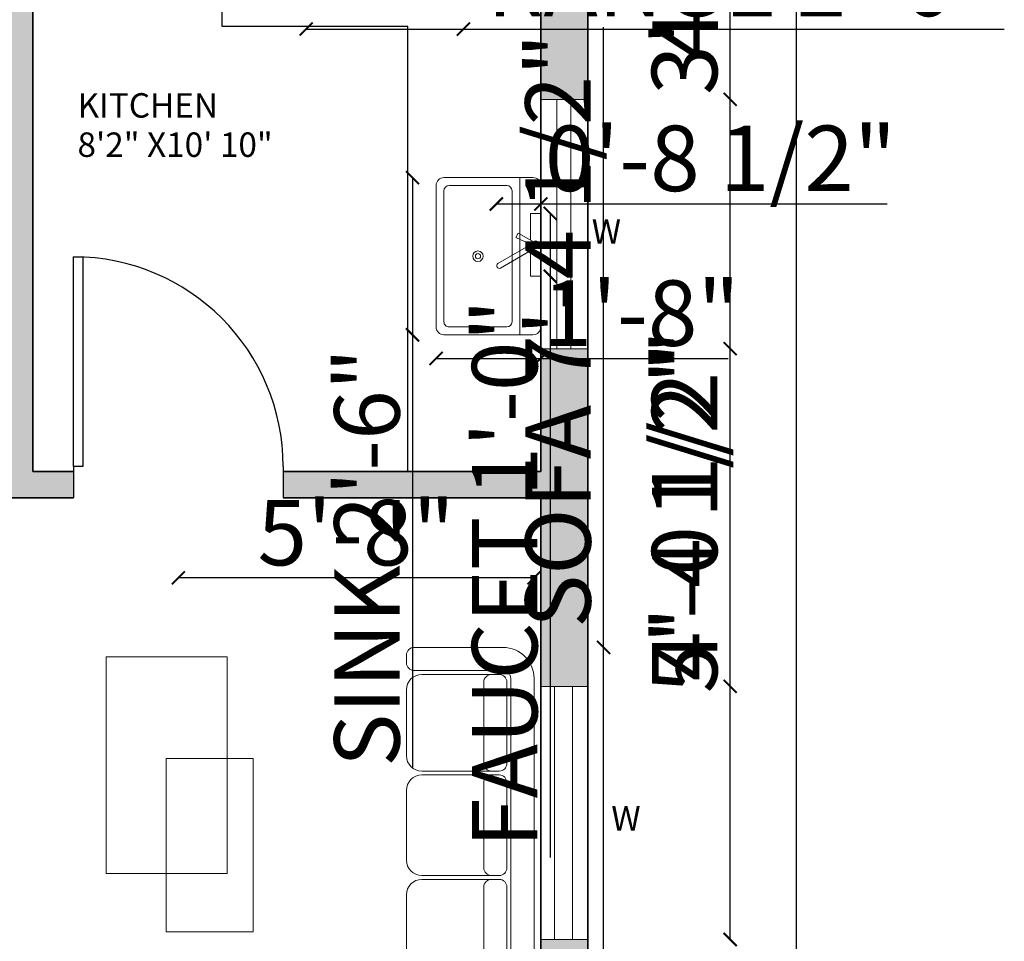
# Model space of a CAD drawing. Units: inches. Extents: x 1750 to 7466, y 1409 to 2004.
# Tile 4 of 5: x 1986 to 2174, y 1715 to 1890. Entities that reach past the tile are written whole.
import ezdxf

# ---------------------------------------------------------------- set-up
doc = ezdxf.new("R2010")
doc.units = ezdxf.units.IN
for name, color, linetype, lineweight in [('A-ANNO-DIMS', 2, 'Continuous', 18), ('A-ANNO-TEXT', 7, 'Continuous', 18), ('A-AREA-IDEN', 7, 'Continuous', 18), ('A-DOOR', 3, 'Continuous', 25), ('A-FLOR-CASE', 8, 'Continuous', 25), ('A-FLOR-FIXT', 9, 'Continuous', 18), ('A-FURN', 8, 'Continuous', 18), ('A-WALL', 7, 'Continuous', 35), ('WINDOW', 4, 'Continuous', 18)]:
    doc.layers.add(name, color=color, linetype=linetype, lineweight=lineweight)
doc.layers.add('A-WALL-PATT', color=18, linetype='Continuous', lineweight=13, true_color=0x000000)
doc.styles.get("Standard").update_dxf_attribs({"font": 'arial.ttf'})
doc.dimstyles.new('ISO-25', dxfattribs={"dimtxt": 12.5, "dimasz": 2.5, "dimexe": 1.25, "dimexo": 0.625, "dimtad": 1, "dimdec": 0, "dimlunit": 4, "dimtxsty": 'Standard', "dimblk": 'ARCHTICK', "dimcen": 2.5, "dimse1": 1, "dimse2": 1, "dimclrd": 2, "dimadec": 0, "dimazin": 0, "dimtfac": 1, "dimtdec": 0, "dimtmove": 0, "dimatfit": 3, "dimfxl": 1, "dimarcsym": 0})

# ---------------------------------------------------------------- blocks, each defined once
blk = doc.blocks.new('A$C2AFA021D')
for p, q in [((0.8, 2.3), (0.2, 2.3)), ((0.85, 2.2), (0.85, 2.25)), ((0.2, 2.15), (0.8, 2.15)), ((0.225, 2.125), (0.275, 2.125)), ((0.75, 2.125), (0.275, 2.125)), ((0, 2.1), (0, 0.2)), ((0.15, 0.2), (0.15, 2.1)), ((0.175, 1.55), (0.175, 2.075)), ((0.325, 2.075), (0.325, 1.55)), ((0.85, 1.6), (0.85, 2.025)), ((0.275, 1.5), (0.225, 1.5)), ((0.225, 1.475), (0.275, 1.475)), ((0.275, 1.5), (0.75, 1.5)), ((0.75, 1.475), (0.275, 1.475)), ((0.175, 0.875), (0.175, 1.425)), ((0.325, 1.425), (0.325, 0.875)), ((0.85, 0.925), (0.85, 1.375)), ((0.275, 0.825), (0.225, 0.825)), ((0.225, 0.8), (0.275, 0.8)), ((0.275, 0.825), (0.75, 0.825)), ((0.75, 0.8), (0.275, 0.8)), ((0.975, 0.825), (1.4, 0.825)), ((1.625, 0.825), (2.075, 0.825)), ((2.3, 0.825), (2.725, 0.825)), ((2.85, 0.2), (2.85, 0.775)), ((2.9, 0.825), (2.95, 0.825)), ((3, 0.775), (3, 0.2)), ((0.175, 0.225), (0.175, 0.75)), ((0.325, 0.75), (0.325, 0.225)), ((0.875, 0.275), (0.875, 0.725)), ((1.5, 0.725), (1.5, 0.275)), ((1.525, 0.275), (1.525, 0.725)), ((2.175, 0.725), (2.175, 0.275)), ((2.2, 0.275), (2.2, 0.725)), ((2.825, 0.725), (2.825, 0.275)), ((0.85, 0.275), (0.85, 0.7)), ((1.45, 0.325), (0.925, 0.325)), ((2.125, 0.325), (1.575, 0.325)), ((2.775, 0.325), (2.25, 0.325)), ((0.875, 0.275), (0.875, 0.225)), ((1.5, 0.225), (1.5, 0.275)), ((1.525, 0.275), (1.525, 0.225)), ((2.175, 0.225), (2.175, 0.275)), ((2.2, 0.275), (2.2, 0.225)), ((2.825, 0.225), (2.825, 0.275)), ((0.8, 0.15), (0.2, 0.15)), ((0.275, 0.175), (0.225, 0.175)), ((0.275, 0.175), (0.75, 0.175)), ((0.925, 0.175), (1.45, 0.175)), ((0.925, 0.15), (2.8, 0.15)), ((1.575, 0.175), (2.125, 0.175)), ((2.25, 0.175), (2.775, 0.175)), ((0.85, 0), (0.85, 0.1)), ((0.875, 0.1), (0.875, 0)), ((0.2, 0), (0.85, 0)), ((2.8, 0), (0.875, 0))]:
    blk.add_line(p, q)
for centre, radius, start, end in [((0.2, 2.1), 0.2, 90, 180), ((0.8, 2.25), 0.05, 0, 90), ((0.8, 2.2), 0.05, 270, 0), ((0.2, 2.1), 0.05, 90, 180), ((0.225, 2.075), 0.05, 90, 180), ((0.275, 2.075), 0.05, 0, 90), ((0.75, 2.025), 0.1, 0, 90), ((0.75, 1.6), 0.1, 270, 0), ((0.225, 1.55), 0.05, 180, 270), ((0.275, 1.55), 0.05, 270, 0), ((0.225, 1.425), 0.05, 90, 180), ((0.275, 1.425), 0.05, 0, 90), ((0.75, 1.375), 0.1, 360, 90), ((0.75, 0.925), 0.1, 270, 0), ((0.225, 0.875), 0.05, 180, 270), ((0.275, 0.875), 0.05, 270, 0), ((0.225, 0.75), 0.05, 90, 180), ((0.275, 0.75), 0.05, 0, 90), ((0.75, 0.7), 0.1, 0, 90), ((0.975, 0.725), 0.1, 90, 180), ((1.4, 0.725), 0.1, 0, 90), ((1.625, 0.725), 0.1, 90, 180), ((2.075, 0.725), 0.1, 0, 90), ((2.3, 0.725), 0.1, 90, 180), ((2.725, 0.725), 0.1, 0, 90), ((2.9, 0.775), 0.05, 90, 180), ((2.95, 0.775), 0.05, 0, 90), ((0.925, 0.275), 0.05, 90, 180), ((1.45, 0.275), 0.05, 360, 90), ((1.575, 0.275), 0.05, 90, 180), ((2.125, 0.275), 0.05, 360, 90), ((2.25, 0.275), 0.05, 90, 180), ((2.775, 0.275), 0.05, 360, 90), ((0.75, 0.275), 0.1, 270, 0), ((0.2, 0.2), 0.2, 180, 270), ((0.2, 0.2), 0.05, 180, 270), ((0.225, 0.225), 0.05, 180, 270), ((0.275, 0.225), 0.05, 270, 0), ((0.925, 0.225), 0.05, 180, 270), ((1.45, 0.225), 0.05, 270, 0), ((1.575, 0.225), 0.05, 180, 270), ((2.125, 0.225), 0.05, 270, 0), ((2.25, 0.225), 0.05, 180, 270), ((2.775, 0.225), 0.05, 270, 0), ((2.8, 0.2), 0.2, 270, 0), ((2.8, 0.2), 0.05, 270, 0), ((0.8, 0.1), 0.05, 0, 90), ((0.925, 0.1), 0.05, 90, 180)]:
    blk.add_arc(centre, radius, start, end)
blk = doc.blocks.new('Faucet - single handle top')
for p, q in [((0.08, -0.26), (-2.26, -4.34)), ((-1.37, -4.79), (0.55, -0.5)), ((4.43, -7.68), (0.72, -1.24)), ((-0.06, -1.9), (3.57, -8.18)), ((-2.26, -4.34), (-1.37, -4.79))]:
    blk.add_line(p, q)
for points in [[(-0.92, -2), (-6, -2), (-6, 0), (6, 0), (6, -2), (1.16, -2)], [(-0.01, -2), (-0.12, -2)]]:
    blk.add_lwpolyline(points)
for centre, radius, start, end in [((0, -1), 0.75, 269.2246, 216.2304), ((4, -7.93), 0.5, 210, 30)]:
    blk.add_arc(centre, radius, start, end)
blk = doc.blocks.new('Sink-single - 30 in top')
blk.add_line((-15, -3.999996), (15, -3.999996))
for points in [[(-13.5, 0), (13.5, 0)], [(-15, -18.499996), (-15, -1.5)], [(15, -1.5), (15, -18.499996)], [(-12.5, -5.499996), (12.5, -5.499996)], [(-13.5, -17.499996), (-13.5, -6.499996)], [(13.5, -6.499996), (13.5, -17.499996)], [(12.5, -18.499996), (-12.5, -18.499996)], [(13.5, -19.999996), (-13.5, -19.999996)]]:
    blk.add_lwpolyline(points)
for radius in [1, 0.5]:
    blk.add_circle((0, -11.999996), radius)
for centre, radius, start, end in [((-13.5, -1.5), 1.5, 90, 180), ((13.5, -1.5), 1.5, 0, 90), ((-12.5, -6.499996), 1, 90, 180), ((12.5, -6.499996), 1, 0, 90), ((-13.5, -18.499996), 1.5, 180, 270), ((-12.5, -17.499996), 1, 180, 270), ((12.5, -17.499996), 1, 270, 0), ((13.5, -18.499996), 1.5, 270, 0)]:
    blk.add_arc(centre, radius, start, end)
blk = doc.blocks.new('*U11')
for p, q in [((0, 0), (0, -6)), ((40, 0), (40, -6))]:
    blk.add_line(p, q)
blk.add_lwpolyline([(0, 0), (0, 40), (1.75, 40), (1.75, 0)], close=True)
blk.add_arc((0, 0), 40, 0, 90)
blk = doc.blocks.new('_ArchTick')
at = {"color": 0, "linetype": 'ByBlock', "const_width": 0.15}
blk.add_lwpolyline([(-0.5, -0.5), (0.5, 0.5)], dxfattribs=at)
blk = doc.blocks.new('*D14')
at = {"layer": 'A-ANNO-DIMS', "color": 0, "lineweight": -2, "transparency": 16777216}
blk.add_line((2133.87, 1928.17), (2133.87, 1448.17), dxfattribs=at)
at = {"layer": 'Defpoints', "color": 0, "transparency": 16777216}
for p in [(2094.13, 1928.17), (2094.13, 1448.17), (2133.87, 1448.17)]:
    blk.add_point(p, dxfattribs=at)
at = {"layer": 'A-ANNO-DIMS', "color": 0, "lineweight": -2, "transparency": 16777216, "xscale": 2.5, "yscale": 2.5, "zscale": 2.5}
for p, rotation in [((2133.87, 1928.17), 90), ((2133.87, 1448.17), 270)]:
    blk.add_blockref('_ArchTick', p, dxfattribs=dict(at, rotation=rotation))
at = {"layer": 'A-ANNO-DIMS', "color": 0, "transparency": 16777216, "insert": (2126.86, 1688.17), "char_height": 12.5, "attachment_point": 5, "rotation": 90}
blk.add_mtext("40'", dxfattribs=at)
blk = doc.blocks.new('*D17')
at = {"layer": 'A-ANNO-DIMS', "color": 2, "lineweight": -2, "transparency": 16777216}
for p, q in [((2097.12, 1770.61), (2097.12, 1889.05)), ((2097.12, 1682.03), (2097.12, 1770.61))]:
    blk.add_line(p, q, dxfattribs=at)
at = {"layer": 'Defpoints', "color": 0, "transparency": 16777216}
for p in [(2083.83, 1770.61), (2097.12, 1770.61), (2083.83, 1682.03)]:
    blk.add_point(p, dxfattribs=at)
at = {"layer": 'A-ANNO-DIMS', "color": 2, "lineweight": -2, "transparency": 16777216, "xscale": 2.5, "yscale": 2.5, "zscale": 2.5}
for p, rotation in [((2097.12, 1770.61), 90), ((2097.12, 1682.03), 270)]:
    blk.add_blockref('_ArchTick', p, dxfattribs=dict(at, rotation=rotation))
at = {"layer": 'A-ANNO-DIMS', "color": 0, "transparency": 16777216, "insert": (2090.03, 1831.08), "char_height": 12.5, "attachment_point": 5, "rotation": 90}
blk.add_mtext('SOFA 7\'-4 1/2"', dxfattribs=at)
blk = doc.blocks.new('*D18')
at = {"layer": 'A-ANNO-DIMS', "color": 2, "lineweight": -2, "transparency": 16777216}
blk.add_line((2083.83, 1783.9), (2015.92, 1783.9), dxfattribs=at)
at = {"layer": 'Defpoints', "color": 0, "transparency": 16777216}
for p in [(2015.92, 1783.9), (2015.92, 1770.61), (2083.83, 1770.61)]:
    blk.add_point(p, dxfattribs=at)
at = {"layer": 'A-ANNO-DIMS', "color": 2, "lineweight": -2, "transparency": 16777216, "xscale": 2.5, "yscale": 2.5, "zscale": 2.5, "rotation": 180}
blk.add_blockref('_ArchTick', (2015.92, 1783.9), dxfattribs=at)
at = {"layer": 'A-ANNO-DIMS', "color": 2, "lineweight": -2, "transparency": 16777216, "xscale": 2.5, "yscale": 2.5, "zscale": 2.5}
blk.add_blockref('_ArchTick', (2083.83, 1783.9), dxfattribs=at)
at = {"layer": 'A-ANNO-DIMS', "color": 0, "transparency": 16777216, "insert": (2049.88, 1790.91), "char_height": 12.5, "attachment_point": 5}
blk.add_mtext('5\'-8"', dxfattribs=at)
blk = doc.blocks.new('*D19')
at = {"layer": 'A-ANNO-DIMS', "color": 2, "lineweight": -2, "transparency": 16777216}
for p, q in [((2040.34, 1888.67), (2070.34, 1888.67)), ((2070.34, 1888.67), (2173.62, 1888.67))]:
    blk.add_line(p, q, dxfattribs=at)
at = {"layer": 'Defpoints', "color": 0, "transparency": 16777216}
for p in [(2040.34, 1893.17), (2070.34, 1893.17), (2070.34, 1888.67)]:
    blk.add_point(p, dxfattribs=at)
at = {"layer": 'A-ANNO-DIMS', "color": 2, "lineweight": -2, "transparency": 16777216, "xscale": 2.5, "yscale": 2.5, "zscale": 2.5, "rotation": 180}
blk.add_blockref('_ArchTick', (2040.34, 1888.67), dxfattribs=at)
at = {"layer": 'A-ANNO-DIMS', "color": 2, "lineweight": -2, "transparency": 16777216, "xscale": 2.5, "yscale": 2.5, "zscale": 2.5}
blk.add_blockref('_ArchTick', (2070.34, 1888.67), dxfattribs=at)
at = {"layer": 'A-ANNO-DIMS', "color": 0, "transparency": 16777216, "insert": (2123.23, 1895.75), "char_height": 12.5, "attachment_point": 5}
blk.add_mtext('RANGE 2\'-6"', dxfattribs=at)
blk = doc.blocks.new('*D21')
at = {"layer": 'A-ANNO-DIMS', "color": 2, "lineweight": -2, "transparency": 16777216}
for p, q in [((2060.63, 1860.3), (2060.63, 1830.3)), ((2060.63, 1830.3), (2060.63, 1747.77))]:
    blk.add_line(p, q, dxfattribs=at)
at = {"layer": 'Defpoints', "color": 0, "transparency": 16777216}
for p in [(2065.13, 1860.3), (2060.63, 1830.3), (2065.13, 1830.3)]:
    blk.add_point(p, dxfattribs=at)
at = {"layer": 'A-ANNO-DIMS', "color": 2, "lineweight": -2, "transparency": 16777216, "xscale": 2.5, "yscale": 2.5, "zscale": 2.5}
for p, rotation in [((2060.63, 1860.3), 90), ((2060.63, 1830.3), 270)]:
    blk.add_blockref('_ArchTick', p, dxfattribs=dict(at, rotation=rotation))
at = {"layer": 'A-ANNO-DIMS', "color": 0, "transparency": 16777216, "insert": (2053.55, 1787.79), "char_height": 12.5, "attachment_point": 5, "rotation": 90}
blk.add_mtext('SINK 2\'-6"', dxfattribs=at)
blk = doc.blocks.new('*D22')
at = {"layer": 'A-ANNO-DIMS', "color": 2, "lineweight": -2, "transparency": 16777216}
for p, q in [((2065.13, 1825.8), (2085.13, 1825.8)), ((2085.13, 1825.8), (2120.93, 1825.8))]:
    blk.add_line(p, q, dxfattribs=at)
at = {"layer": 'Defpoints', "color": 0, "transparency": 16777216}
for p in [(2065.13, 1830.3), (2085.13, 1830.3), (2085.13, 1825.8)]:
    blk.add_point(p, dxfattribs=at)
at = {"layer": 'A-ANNO-DIMS', "color": 2, "lineweight": -2, "transparency": 16777216, "xscale": 2.5, "yscale": 2.5, "zscale": 2.5, "rotation": 180}
blk.add_blockref('_ArchTick', (2065.13, 1825.8), dxfattribs=at)
at = {"layer": 'A-ANNO-DIMS', "color": 2, "lineweight": -2, "transparency": 16777216, "xscale": 2.5, "yscale": 2.5, "zscale": 2.5}
blk.add_blockref('_ArchTick', (2085.13, 1825.8), dxfattribs=at)
at = {"layer": 'A-ANNO-DIMS', "color": 0, "transparency": 16777216, "insert": (2104.28, 1832.81), "char_height": 12.5, "attachment_point": 5}
blk.add_mtext('1\'-8"', dxfattribs=at)
blk = doc.blocks.new('*D23')
at = {"layer": 'A-ANNO-DIMS', "color": 2, "lineweight": -2, "transparency": 16777216}
for p, q in [((2086.93, 1853.47), (2086.93, 1841.47)), ((2086.93, 1841.47), (2086.93, 1730.5))]:
    blk.add_line(p, q, dxfattribs=at)
at = {"layer": 'Defpoints', "color": 0, "transparency": 16777216}
for p in [(2085.13, 1853.47), (2085.13, 1841.47), (2086.93, 1841.47)]:
    blk.add_point(p, dxfattribs=at)
at = {"layer": 'A-ANNO-DIMS', "color": 2, "lineweight": -2, "transparency": 16777216, "xscale": 2.5, "yscale": 2.5, "zscale": 2.5}
for p, rotation in [((2086.93, 1853.47), 90), ((2086.93, 1841.47), 270)]:
    blk.add_blockref('_ArchTick', p, dxfattribs=dict(at, rotation=rotation))
at = {"layer": 'A-ANNO-DIMS', "color": 0, "transparency": 16777216, "insert": (2079.85, 1784.74), "char_height": 12.5, "attachment_point": 5, "rotation": 90}
blk.add_mtext('FAUCET 1\'-0"', dxfattribs=at)
blk = doc.blocks.new('*D24')
at = {"layer": 'A-ANNO-DIMS', "color": 2, "lineweight": -2, "transparency": 16777216}
for p, q in [((2076.63, 1855.27), (2085.13, 1855.27)), ((2085.13, 1855.27), (2151.24, 1855.27))]:
    blk.add_line(p, q, dxfattribs=at)
at = {"layer": 'Defpoints', "color": 0, "transparency": 16777216}
for p in [(2085.13, 1855.27), (2076.63, 1853.47), (2085.13, 1853.47)]:
    blk.add_point(p, dxfattribs=at)
at = {"layer": 'A-ANNO-DIMS', "color": 2, "lineweight": -2, "transparency": 16777216, "xscale": 2.5, "yscale": 2.5, "zscale": 2.5, "rotation": 180}
blk.add_blockref('_ArchTick', (2076.63, 1855.27), dxfattribs=at)
at = {"layer": 'A-ANNO-DIMS', "color": 2, "lineweight": -2, "transparency": 16777216, "xscale": 2.5, "yscale": 2.5, "zscale": 2.5}
blk.add_blockref('_ArchTick', (2085.13, 1855.27), dxfattribs=at)
at = {"layer": 'A-ANNO-DIMS', "color": 0, "transparency": 16777216, "insert": (2119.44, 1862.36), "char_height": 12.5, "attachment_point": 5}
blk.add_mtext('0\'-8 1/2"', dxfattribs=at)
blk = doc.blocks.new('*D38')
at = {"layer": 'A-ANNO-DIMS', "color": 2, "lineweight": -2, "transparency": 16777216}
for p, q in [((2024.28, 1421.02), (2059.72, 1421.02)), ((2059.72, 1421.02), (2135.75, 1421.02))]:
    blk.add_line(p, q, dxfattribs=at)
at = {"layer": 'Defpoints', "color": 0, "transparency": 16777216}
for p in [(2024.28, 1889.13), (2059.72, 1889.13), (2059.72, 1421.02)]:
    blk.add_point(p, dxfattribs=at)
at = {"layer": 'A-ANNO-DIMS', "color": 2, "lineweight": -2, "transparency": 16777216, "xscale": 2.5, "yscale": 2.5, "zscale": 2.5, "rotation": 180}
blk.add_blockref('_ArchTick', (2024.28, 1421.02), dxfattribs=at)
at = {"layer": 'A-ANNO-DIMS', "color": 2, "lineweight": -2, "transparency": 16777216, "xscale": 2.5, "yscale": 2.5, "zscale": 2.5}
blk.add_blockref('_ArchTick', (2059.72, 1421.02), dxfattribs=at)
at = {"layer": 'A-ANNO-DIMS', "color": 0, "transparency": 16777216, "insert": (2098.98, 1428.1), "char_height": 12.5, "attachment_point": 5}
blk.add_mtext('2\'-11 1/2"', dxfattribs=at)
blk = doc.blocks.new('*D39')
at = {"layer": 'A-ANNO-DIMS', "color": 2, "lineweight": -2, "transparency": 16777216}
for p, q in [((1775.98, 1919.17), (1775.98, 1889.13)), ((1775.98, 1889.13), (1775.98, 1851.94))]:
    blk.add_line(p, q, dxfattribs=at)
at = {"layer": 'Defpoints', "color": 0, "transparency": 16777216}
for p in [(2024.28, 1919.17), (1775.98, 1889.13), (2024.28, 1889.13)]:
    blk.add_point(p, dxfattribs=at)
at = {"layer": 'A-ANNO-DIMS', "color": 2, "lineweight": -2, "transparency": 16777216, "xscale": 2.5, "yscale": 2.5, "zscale": 2.5}
for p, rotation in [((1775.98, 1919.17), 90), ((1775.98, 1889.13), 270)]:
    blk.add_blockref('_ArchTick', p, dxfattribs=dict(at, rotation=rotation))
at = {"layer": 'A-ANNO-DIMS', "color": 0, "transparency": 16777216, "insert": (1768.98, 1869.28), "char_height": 12.5, "attachment_point": 5, "rotation": 90}
blk.add_mtext('2\'-6"', dxfattribs=at)
blk = doc.blocks.new('*D40')
at = {"layer": 'A-ANNO-DIMS', "color": 2, "lineweight": -2, "transparency": 16777216}
for p, q in [((2059.72, 1421.02), (2085.13, 1421.02)), ((2085.13, 1421.02), (2151.45, 1421.02))]:
    blk.add_line(p, q, dxfattribs=at)
at = {"layer": 'Defpoints', "color": 0, "transparency": 16777216}
for p in [(2059.72, 1804.17), (2085.13, 1804.17), (2085.13, 1421.02)]:
    blk.add_point(p, dxfattribs=at)
at = {"layer": 'A-ANNO-DIMS', "color": 2, "lineweight": -2, "transparency": 16777216, "xscale": 2.5, "yscale": 2.5, "zscale": 2.5, "rotation": 180}
blk.add_blockref('_ArchTick', (2059.72, 1421.02), dxfattribs=at)
at = {"layer": 'A-ANNO-DIMS', "color": 2, "lineweight": -2, "transparency": 16777216, "xscale": 2.5, "yscale": 2.5, "zscale": 2.5}
blk.add_blockref('_ArchTick', (2085.13, 1421.02), dxfattribs=at)
at = {"layer": 'A-ANNO-DIMS', "color": 0, "transparency": 16777216, "insert": (2119.54, 1428.1), "char_height": 12.5, "attachment_point": 5}
blk.add_mtext('2\'-1 1/2"', dxfattribs=at)
blk = doc.blocks.new('*D41')
at = {"layer": 'A-ANNO-DIMS', "color": 2, "lineweight": -2, "transparency": 16777216}
blk.add_line((1995.93, 1421.02), (2035.93, 1421.02), dxfattribs=at)
at = {"layer": 'Defpoints', "color": 0, "transparency": 16777216}
for p in [(1995.93, 1804.17), (2035.93, 1804.17), (2035.93, 1421.02)]:
    blk.add_point(p, dxfattribs=at)
at = {"layer": 'A-ANNO-DIMS', "color": 2, "lineweight": -2, "transparency": 16777216, "xscale": 2.5, "yscale": 2.5, "zscale": 2.5, "rotation": 180}
blk.add_blockref('_ArchTick', (1995.93, 1421.02), dxfattribs=at)
at = {"layer": 'A-ANNO-DIMS', "color": 2, "lineweight": -2, "transparency": 16777216, "xscale": 2.5, "yscale": 2.5, "zscale": 2.5}
blk.add_blockref('_ArchTick', (2035.93, 1421.02), dxfattribs=at)
at = {"layer": 'A-ANNO-DIMS', "color": 0, "transparency": 16777216, "insert": (2015.93, 1428.03), "char_height": 12.5, "attachment_point": 5}
blk.add_mtext('3\'-4"', dxfattribs=at)
blk = doc.blocks.new('*D44')
at = {"layer": 'A-ANNO-DIMS', "color": 2, "lineweight": -2, "transparency": 16777216}
for p, q in [((2121.28, 1875.24), (2121.28, 1951.04)), ((2121.28, 1827.64), (2121.28, 1875.24))]:
    blk.add_line(p, q, dxfattribs=at)
at = {"layer": 'Defpoints', "color": 0, "transparency": 16777216}
for p in [(2094.13, 1875.24), (2121.28, 1875.24), (2094.13, 1827.64)]:
    blk.add_point(p, dxfattribs=at)
at = {"layer": 'A-ANNO-DIMS', "color": 2, "lineweight": -2, "transparency": 16777216, "xscale": 2.5, "yscale": 2.5, "zscale": 2.5}
for p, rotation in [((2121.28, 1875.24), 90), ((2121.28, 1827.64), 270)]:
    blk.add_blockref('_ArchTick', p, dxfattribs=dict(at, rotation=rotation))
at = {"layer": 'A-ANNO-DIMS', "color": 0, "transparency": 16777216, "insert": (2114.19, 1914.39), "char_height": 12.5, "attachment_point": 5, "rotation": 90}
blk.add_mtext('3\'-11 1/2"', dxfattribs=at)
blk = doc.blocks.new('*D45')
at = {"layer": 'A-ANNO-DIMS', "color": 2, "lineweight": -2, "transparency": 16777216}
blk.add_line((2121.28, 1875.24), (2121.28, 1928.17), dxfattribs=at)
at = {"layer": 'Defpoints', "color": 0, "transparency": 16777216}
for p in [(2094.13, 1928.17), (2121.28, 1928.17), (2094.13, 1875.24)]:
    blk.add_point(p, dxfattribs=at)
at = {"layer": 'A-ANNO-DIMS', "color": 2, "lineweight": -2, "transparency": 16777216, "xscale": 2.5, "yscale": 2.5, "zscale": 2.5}
for p, rotation in [((2121.28, 1928.17), 90), ((2121.28, 1875.24), 270)]:
    blk.add_blockref('_ArchTick', p, dxfattribs=dict(at, rotation=rotation))
at = {"layer": 'A-ANNO-DIMS', "color": 0, "transparency": 16777216, "insert": (2114.3, 1901.7), "char_height": 12.5, "attachment_point": 5, "rotation": 90}
blk.add_mtext('4\'-5"', dxfattribs=at)
blk = doc.blocks.new('*D46')
at = {"layer": 'A-ANNO-DIMS', "color": 2, "lineweight": -2, "transparency": 16777216}
for p, q in [((1775.98, 1830.3), (1775.98, 1804.17)), ((1775.98, 1804.17), (1775.98, 1766.97))]:
    blk.add_line(p, q, dxfattribs=at)
at = {"layer": 'Defpoints', "color": 0, "transparency": 16777216}
for p in [(2066.63, 1830.3), (1775.98, 1804.17), (2059.72, 1804.17)]:
    blk.add_point(p, dxfattribs=at)
at = {"layer": 'A-ANNO-DIMS', "color": 2, "lineweight": -2, "transparency": 16777216, "xscale": 2.5, "yscale": 2.5, "zscale": 2.5}
for p, rotation in [((1775.98, 1830.3), 90), ((1775.98, 1804.17), 270)]:
    blk.add_blockref('_ArchTick', p, dxfattribs=dict(at, rotation=rotation))
at = {"layer": 'A-ANNO-DIMS', "color": 0, "transparency": 16777216, "insert": (1769.08, 1784.32), "char_height": 12.5, "attachment_point": 5, "rotation": 90}
blk.add_mtext('2\'-2"', dxfattribs=at)
blk = doc.blocks.new('*D47')
at = {"layer": 'A-ANNO-DIMS', "color": 2, "lineweight": -2, "transparency": 16777216}
for p, q in [((1775.98, 1928.17), (1775.98, 1919.17)), ((1775.98, 1919.17), (1775.98, 1882.19))]:
    blk.add_line(p, q, dxfattribs=at)
at = {"layer": 'Defpoints', "color": 0, "transparency": 16777216}
for p in [(2022.32, 1928.17), (1775.98, 1919.17), (2022.32, 1919.17)]:
    blk.add_point(p, dxfattribs=at)
at = {"layer": 'A-ANNO-DIMS', "color": 2, "lineweight": -2, "transparency": 16777216, "xscale": 2.5, "yscale": 2.5, "zscale": 2.5}
for p, rotation in [((1775.98, 1928.17), 90), ((1775.98, 1919.17), 270)]:
    blk.add_blockref('_ArchTick', p, dxfattribs=dict(at, rotation=rotation))
at = {"layer": 'A-ANNO-DIMS', "color": 0, "transparency": 16777216, "insert": (1768.98, 1899.43), "char_height": 12.5, "attachment_point": 5, "rotation": 90}
blk.add_mtext('0\'-9"', dxfattribs=at)
blk = doc.blocks.new('*D48')
at = {"layer": 'A-ANNO-DIMS', "color": 2, "lineweight": -2, "transparency": 16777216}
for p, q in [((1983.13, 1421.02), (1988.13, 1421.02)), ((1988.13, 1421.02), (2025.11, 1421.02))]:
    blk.add_line(p, q, dxfattribs=at)
at = {"layer": 'Defpoints', "color": 0, "transparency": 16777216}
for p in [(1983.13, 1804.17), (1988.13, 1804.17), (1988.13, 1421.02)]:
    blk.add_point(p, dxfattribs=at)
at = {"layer": 'A-ANNO-DIMS', "color": 2, "lineweight": -2, "transparency": 16777216, "xscale": 2.5, "yscale": 2.5, "zscale": 2.5, "rotation": 180}
blk.add_blockref('_ArchTick', (1983.13, 1421.02), dxfattribs=at)
at = {"layer": 'A-ANNO-DIMS', "color": 2, "lineweight": -2, "transparency": 16777216, "xscale": 2.5, "yscale": 2.5, "zscale": 2.5}
blk.add_blockref('_ArchTick', (1988.13, 1421.02), dxfattribs=at)
at = {"layer": 'A-ANNO-DIMS', "color": 0, "transparency": 16777216, "insert": (2007.87, 1428.02), "char_height": 12.5, "attachment_point": 5}
blk.add_mtext('0\'-5"', dxfattribs=at)
blk = doc.blocks.new('*D53')
at = {"layer": 'A-ANNO-DIMS', "color": 2, "lineweight": -2, "transparency": 16777216}
for p, q in [((2121.28, 1763.18), (2121.28, 1829.79)), ((2121.28, 1714.84), (2121.28, 1763.18))]:
    blk.add_line(p, q, dxfattribs=at)
at = {"layer": 'Defpoints', "color": 0, "transparency": 16777216}
for p in [(2094.13, 1763.18), (2121.28, 1763.18), (2094.13, 1714.84)]:
    blk.add_point(p, dxfattribs=at)
at = {"layer": 'A-ANNO-DIMS', "color": 2, "lineweight": -2, "transparency": 16777216, "xscale": 2.5, "yscale": 2.5, "zscale": 2.5}
for p, rotation in [((2121.28, 1763.18), 90), ((2121.28, 1714.84), 270)]:
    blk.add_blockref('_ArchTick', p, dxfattribs=dict(at, rotation=rotation))
at = {"layer": 'A-ANNO-DIMS', "color": 0, "transparency": 16777216, "insert": (2114.2, 1797.73), "char_height": 12.5, "attachment_point": 5, "rotation": 90}
blk.add_mtext('4\'-0 1/2"', dxfattribs=at)
blk = doc.blocks.new('*D54')
at = {"layer": 'A-ANNO-DIMS', "color": 2, "lineweight": -2, "transparency": 16777216}
blk.add_line((2121.28, 1763.18), (2121.28, 1827.64), dxfattribs=at)
at = {"layer": 'Defpoints', "color": 0, "transparency": 16777216}
for p in [(2094.13, 1827.64), (2121.28, 1827.64), (2094.13, 1763.18)]:
    blk.add_point(p, dxfattribs=at)
at = {"layer": 'A-ANNO-DIMS', "color": 2, "lineweight": -2, "transparency": 16777216, "xscale": 2.5, "yscale": 2.5, "zscale": 2.5}
for p, rotation in [((2121.28, 1827.64), 90), ((2121.28, 1763.18), 270)]:
    blk.add_blockref('_ArchTick', p, dxfattribs=dict(at, rotation=rotation))
at = {"layer": 'A-ANNO-DIMS', "color": 0, "transparency": 16777216, "insert": (2114.2, 1795.41), "char_height": 12.5, "attachment_point": 5, "rotation": 90}
blk.add_mtext('5\'-4 1/2"', dxfattribs=at)
blk = doc.blocks.new('*D55')
at = {"layer": 'A-ANNO-DIMS', "color": 2, "lineweight": -2, "transparency": 16777216}
blk.add_line((1775.98, 1928.17), (1775.98, 1799.17), dxfattribs=at)
at = {"layer": 'Defpoints', "color": 0, "transparency": 16777216}
for p in [(2022.32, 1928.17), (1775.98, 1799.17), (1995.93, 1799.17)]:
    blk.add_point(p, dxfattribs=at)
at = {"layer": 'A-ANNO-DIMS', "color": 2, "lineweight": -2, "transparency": 16777216, "xscale": 2.5, "yscale": 2.5, "zscale": 2.5}
for p, rotation in [((1775.98, 1928.17), 90), ((1775.98, 1799.17), 270)]:
    blk.add_blockref('_ArchTick', p, dxfattribs=dict(at, rotation=rotation))
at = {"layer": 'A-ANNO-DIMS', "color": 0, "transparency": 16777216, "insert": (1768.98, 1863.67), "char_height": 12.5, "attachment_point": 5, "rotation": 90}
blk.add_mtext('10\'-9"', dxfattribs=at)

msp = doc.modelspace()

# ---------------------------------------------------------------- hatches: boundary and pattern name
at = {"layer": 'A-WALL-PATT'}
h = msp.add_hatch(color=256, dxfattribs=at)
h.dxf.hatch_style = 1
h.paths.add_polyline_path([(1896.49, 1928.17), (1854.13, 1928.17), (1854.13, 1893.52), (1863.13, 1893.52), (1863.13, 1919.17), (1896.49, 1919.17)])
h.paths.add_polyline_path([(2022.32, 1928.17), (1945.82, 1928.17), (1945.82, 1919.17), (1983.13, 1919.17), (1983.13, 1804.17), (1974.13, 1804.17), (1974.13, 1799.17), (1995.93, 1799.17), (1995.93, 1804.17), (1988.13, 1804.17), (1988.13, 1919.17), (2022.32, 1919.17)])
h.paths.add_polyline_path([(2094.13, 1928.17), (2070.34, 1928.17), (2070.34, 1919.17), (2085.13, 1919.17), (2085.13, 1875.24), (2094.13, 1875.24)])
h.paths.add_polyline_path([(2094.13, 1827.64), (2085.13, 1827.64), (2085.13, 1804.17), (2035.93, 1804.17), (2035.93, 1799.17), (2085.13, 1799.17), (2085.13, 1763.18), (2094.13, 1763.18)])
h.paths.add_polyline_path([(1863.13, 1846.52), (1854.13, 1846.52), (1854.13, 1751.88), (1863.13, 1751.88)])
h.paths.add_polyline_path([(1934.13, 1804.17), (1863.13, 1804.17), (1863.13, 1799.17), (1911.13, 1799.17), (1911.13, 1794.68), (1912.55, 1794.68), (1916.13, 1794.68), (1916.13, 1799.17), (1934.13, 1799.17)])
h.paths.add_polyline_path([(1863.13, 1726.23), (1854.13, 1726.23), (1854.13, 1709.82), (1863.13, 1709.82), (1863.13, 1714.17), (1911.13, 1714.17), (1911.13, 1671.17), (1887.9, 1671.17, -0.01479), (1887.95, 1669.75), (1887.95, 1666.17), (1916.13, 1666.17), (1940.64, 1666.17), (1940.64, 1671.17), (1916.13, 1671.17), (1916.13, 1770.77), (1912.55, 1770.77, -0.01479), (1911.13, 1770.81), (1911.13, 1719.17), (1863.13, 1719.17)])
h.paths.add_polyline_path([(1863.13, 1684.17), (1854.13, 1684.17), (1854.13, 1625.24), (1863.13, 1625.24)])
h.paths.add_polyline_path([(1863.13, 1577.33), (1854.13, 1577.33), (1854.13, 1526.31), (1863.13, 1526.31), (1863.13, 1544.17), (1983.13, 1544.17), (1988.13, 1544.17), (1990.13, 1544.17), (1990.13, 1549.17), (1990.13, 1620.17), (1996.77, 1620.17), (1996.77, 1625.17), (1990.13, 1625.17), (1990.13, 1666.17), (1990.13, 1671.17), (1980.64, 1671.17), (1980.64, 1666.17), (1985.13, 1666.17), (1985.13, 1625.17), (1985.13, 1549.17), (1863.13, 1549.17)])
h.paths.add_polyline_path([(1988.13, 1457.17), (1863.13, 1457.17), (1863.13, 1497.36), (1854.13, 1497.36), (1854.13, 1448.17), (1988.13, 1448.17)])
h.paths.add_polyline_path([(2031.23, 1454.78), (1988.13, 1454.78), (1988.13, 1450.91), (2031.23, 1450.91)])
h.paths.add_polyline_path([(2074.33, 1454.78), (2037.79, 1454.78), (2037.79, 1450.91), (2074.33, 1450.91)], flags=17)
h.paths.add_polyline_path([(2094.13, 1714.84), (2085.13, 1714.84), (2085.13, 1625.17), (2036.77, 1625.17), (2036.77, 1620.17), (2085.13, 1620.17), (2085.13, 1457.17), (2074.33, 1457.17), (2074.33, 1448.17), (2094.13, 1448.17)])
h.paths.add_polyline_path([(1846.92, 1867), (1855.4, 1867), (1855.4, 1874), (1846.92, 1874)], flags=9)
h.paths.add_polyline_path([(1885.75, 1686.15), (1909.97, 1686.15), (1909.97, 1693.31), (1885.75, 1693.31)], flags=25)
h.paths.add_polyline_path([(1885.73, 1693.64), (1900.82, 1693.64), (1900.82, 1700.88), (1885.73, 1700.88)], flags=25)
h.paths.add_polyline_path([(1866.42, 1762.99), (1892.45, 1762.99), (1892.45, 1770.14), (1866.42, 1770.14)], flags=25)
h.paths.add_polyline_path([(1866.4, 1770.47), (1898.87, 1770.47), (1898.87, 1777.71), (1866.4, 1777.71)], flags=9)
h.paths.add_polyline_path([(1925.02, 1731.07), (1964.24, 1731.07), (1964.24, 1738.22), (1925.02, 1738.22)], flags=9)
h.paths.add_polyline_path([(1925.01, 1738.55), (1982.11, 1738.55), (1982.11, 1745.79), (1925.01, 1745.79)], flags=9)
h.paths.add_polyline_path([(1995.48, 1862.99), (2034.71, 1862.99), (2034.71, 1870.14), (1995.48, 1870.14)], flags=9)
h.paths.add_polyline_path([(1995.47, 1870.47), (2026.49, 1870.47), (2026.49, 1877.71), (1995.47, 1877.71)], flags=9)
h.paths.add_polyline_path([(1869.07, 1829.02), (1905.98, 1829.02), (1905.98, 1836.17), (1869.07, 1836.17)], flags=9)
h.paths.add_polyline_path([(1869.05, 1836.5), (1905.15, 1836.5), (1905.15, 1843.74), (1869.05, 1843.74)], flags=9)

# ---------------------------------------------------------------- linework, layer by layer
at = {"layer": 'A-FLOR-CASE'}
for p, q in [((2024.28, 1889.13), (2024.28, 1919.17)), ((2059.72, 1889.13), (2024.28, 1889.13)), ((2059.72, 1804.17), (2059.72, 1889.13))]:
    msp.add_line(p, q, dxfattribs=at)
at = {"layer": 'A-FURN'}
for points in [[(2002.13, 1768.84), (2025.25, 1768.84), (2025.25, 1727.45), (2002.13, 1727.45)], [(2013.58, 1749.38), (2030.2, 1749.38), (2030.2, 1716.32), (2013.58, 1716.32)]]:
    msp.add_lwpolyline(points, close=True, dxfattribs=at)
at = {"layer": 'A-WALL'}
for p, q in [((1988.13, 1804.17), (1988.13, 1919.17)), ((2085.13, 1919.17), (2085.13, 1804.17)), ((1988.13, 1804.17), (1995.93, 1804.17)), ((2035.93, 1804.17), (2085.13, 1804.17)), ((1974.13, 1799.17), (1995.93, 1799.17)), ((2035.93, 1799.17), (2085.13, 1799.17)), ((2085.13, 1799.17), (2085.13, 1625.17))]:
    msp.add_line(p, q, dxfattribs=at)
msp.add_lwpolyline([(1988.13, 1448.17), (1854.13, 1448.17), (1854.13, 1928.17), (2094.13, 1928.17), (2094.13, 1448.17), (2074.33, 1448.17)], dxfattribs=at)
at = {"layer": 'WINDOW'}
for p, q in [((2094.13, 1875.24), (2085.13, 1875.24)), ((2085.13, 1875.24), (2085.13, 1827.64)), ((2088.16, 1827.64), (2088.16, 1875.24)), ((2090.84, 1827.64), (2090.84, 1875.24)), ((2094.13, 1827.64), (2094.13, 1875.24)), ((2085.13, 1827.64), (2094.13, 1827.64)), ((2094.13, 1763.18), (2085.13, 1763.18)), ((2085.13, 1763.18), (2085.13, 1714.84)), ((2087.75, 1714.84), (2087.75, 1763.18)), ((2091.19, 1714.84), (2091.19, 1763.18)), ((2094.13, 1714.84), (2094.13, 1763.18)), ((2085.13, 1714.84), (2094.13, 1714.84))]:
    msp.add_line(p, q, dxfattribs=at)

# ---------------------------------------------------------------- block references
at = {"layer": 'A-DOOR'}
msp.add_blockref('*U11', (1995.93, 1805.17), dxfattribs=at)
at = {"layer": 'A-FLOR-FIXT', "rotation": 270}
for name, p in [('Sink-single - 30 in top', (2085.13, 1845.3)), ('Faucet - single handle top', (2085.13, 1847.47))]:
    msp.add_blockref(name, p, dxfattribs=at)
at = {"layer": 'A-FURN', "xscale": 29.52853756539839, "yscale": 29.52853756539839, "zscale": 29.52853756539839, "rotation": 90}
msp.add_blockref('A$C2AFA021D', (2083.83, 1682.03), dxfattribs=at)

# ---------------------------------------------------------------- texts
at = {"layer": 'A-ANNO-TEXT'}
for p in [(2094.85, 1847.69), (2098.59, 1735.65)]:
    msp.add_text('W', height=4.67, dxfattribs=at).set_placement(p)
at = {"layer": 'A-AREA-IDEN'}
for s, height, p in [('KITCHEN', 4.666, (1996.67, 1871.76)), ('8\'2" X10\' 10"', 4.6662, (1996.67, 1864.26))]:
    msp.add_text(s, height=height, dxfattribs=at).set_placement(p)

# ---------------------------------------------------------------- dimensions: what is measured, and where the dimension line sits
at = {"layer": 'A-ANNO-DIMS'}
for base, p1, p2, angle, override, picture, middle in [((2121.28, 1875.24), (2094.13, 1827.64), (2094.13, 1875.24), 90, {"dimdec": 1, "dimlfac": 1, "dimrnd": 0, "dimzin": 1, "dimdsep": 46, "dimlunit": 4, "dimfrac": 2}, '*D44', (2114.19, 1914.39)), ((1775.98, 1919.17), (2022.32, 1928.17), (2022.32, 1919.17), 90, {"dimdec": 1, "dimlfac": 1, "dimrnd": 0, "dimzin": 1, "dimdsep": 46, "dimlunit": 4, "dimfrac": 2}, '*D47', (1768.98, 1899.43)), ((1775.98, 1799.17), (2022.32, 1928.17), (1995.93, 1799.17), 90, {"dimdec": 1, "dimlfac": 1, "dimrnd": 0, "dimzin": 1, "dimdsep": 46, "dimlunit": 4, "dimfrac": 2}, '*D55', (1768.98, 1863.67)), ((2133.87, 1448.17), (2094.13, 1928.17), (2094.13, 1448.17), 90, {"dimclrd": 0, "dimclre": 0, "dimclrt": 0}, '*D14', (2126.86, 1688.17)), ((2121.28, 1928.17), (2094.13, 1875.24), (2094.13, 1928.17), 90, {"dimdec": 1, "dimlfac": 1, "dimrnd": 0, "dimzin": 1, "dimdsep": 46, "dimlunit": 4, "dimfrac": 2}, '*D45', (2114.3, 1901.7)), ((1775.98, 1889.13), (2024.28, 1919.17), (2024.28, 1889.13), 90, {"dimdec": 1, "dimlfac": 1, "dimrnd": 0, "dimzin": 1, "dimdsep": 46, "dimlunit": 4, "dimfrac": 2}, '*D39', (1768.98, 1869.28)), ((1775.98, 1804.17), (2066.63, 1830.3), (2059.72, 1804.17), 90, {"dimdec": 1, "dimlfac": 1, "dimrnd": 0, "dimzin": 1, "dimdsep": 46, "dimlunit": 4, "dimfrac": 2}, '*D46', (1769.08, 1784.32)), ((2121.28, 1763.18), (2094.13, 1714.84), (2094.13, 1763.18), 90, {"dimdec": 1, "dimlfac": 1, "dimrnd": 0, "dimzin": 1, "dimdsep": 46, "dimlunit": 4, "dimfrac": 2}, '*D53', (2114.2, 1797.73)), ((2121.28, 1827.64), (2094.13, 1763.18), (2094.13, 1827.64), 90, {"dimdec": 1, "dimlfac": 1, "dimrnd": 0, "dimzin": 1, "dimdsep": 46, "dimlunit": 4, "dimfrac": 2}, '*D54', (2114.2, 1795.41)), ((2015.92, 1783.9), (2083.83, 1770.61), (2015.92, 1770.61), 180, {"dimdec": 1, "dimlfac": 1, "dimrnd": 0, "dimzin": 1, "dimdsep": 46, "dimlunit": 4, "dimfrac": 2}, '*D18', (2049.88, 1790.91))]:
    dim = msp.add_linear_dim(base=base, p1=p1, p2=p2, angle=angle, dimstyle='ISO-25', override=override, dxfattribs=at)
    dim.commit()
    dim.dimension.update_dxf_attribs({"geometry": picture, "text_midpoint": middle})
dim = msp.add_linear_dim(base=(2070.34, 1888.67), p1=(2040.34, 1893.17), p2=(2070.34, 1893.17), text='RANGE <>', dimstyle='ISO-25', override={"dimdec": 1, "dimlfac": 1, "dimrnd": 0, "dimzin": 1, "dimdsep": 46, "dimlunit": 4, "dimfrac": 2}, dxfattribs=at)
dim.commit()
dim.dimension.update_dxf_attribs({"geometry": '*D19', "text_midpoint": (2123.23, 1895.75)})
for base, p1, p2, picture, middle in [((2059.72, 1421.02), (2024.28, 1889.13), (2059.72, 1889.13), '*D38', (2098.98, 1428.1)), ((2085.13, 1855.27), (2076.63, 1853.47), (2085.13, 1853.47), '*D24', (2119.44, 1862.36)), ((2085.13, 1825.8), (2065.13, 1830.3), (2085.13, 1830.3), '*D22', (2104.28, 1832.81)), ((1988.13, 1421.02), (1983.13, 1804.17), (1988.13, 1804.17), '*D48', (2007.87, 1428.02)), ((2035.93, 1421.02), (1995.93, 1804.17), (2035.93, 1804.17), '*D41', (2015.93, 1428.03)), ((2085.13, 1421.02), (2059.72, 1804.17), (2085.13, 1804.17), '*D40', (2119.54, 1428.1))]:
    dim = msp.add_linear_dim(base=base, p1=p1, p2=p2, dimstyle='ISO-25', override={"dimdec": 1, "dimlfac": 1, "dimrnd": 0, "dimzin": 1, "dimdsep": 46, "dimlunit": 4, "dimfrac": 2}, dxfattribs=at)
    dim.commit()
    dim.dimension.update_dxf_attribs({"geometry": picture, "text_midpoint": middle})
for base, p1, p2, angle, text, picture, middle in [((2097.12, 1770.61), (2083.83, 1682.03), (2083.83, 1770.61), 90, 'SOFA <>', '*D17', (2090.03, 1831.08)), ((2060.63, 1830.3), (2065.13, 1860.3), (2065.13, 1830.3), 270, 'SINK <>', '*D21', (2053.55, 1787.79)), ((2086.93, 1841.47), (2085.13, 1853.47), (2085.13, 1841.47), 270, 'FAUCET <>', '*D23', (2079.85, 1784.74))]:
    dim = msp.add_linear_dim(base=base, p1=p1, p2=p2, angle=angle, text=text, dimstyle='ISO-25', override={"dimdec": 1, "dimlfac": 1, "dimrnd": 0, "dimzin": 1, "dimdsep": 46, "dimlunit": 4, "dimfrac": 2}, dxfattribs=at)
    dim.commit()
    dim.dimension.update_dxf_attribs({"geometry": picture, "text_midpoint": middle})

doc.saveas('drawing.dxf')
